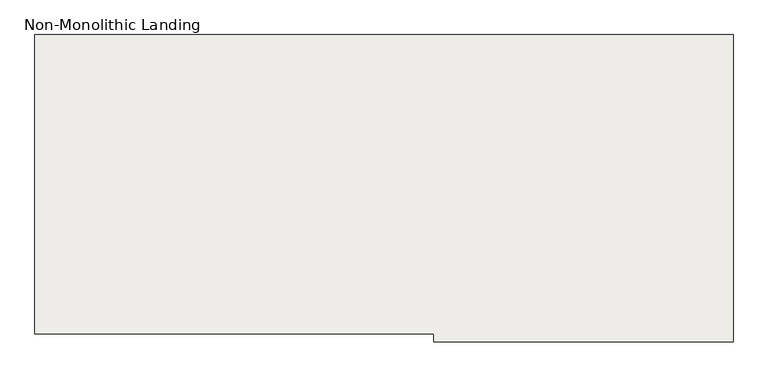
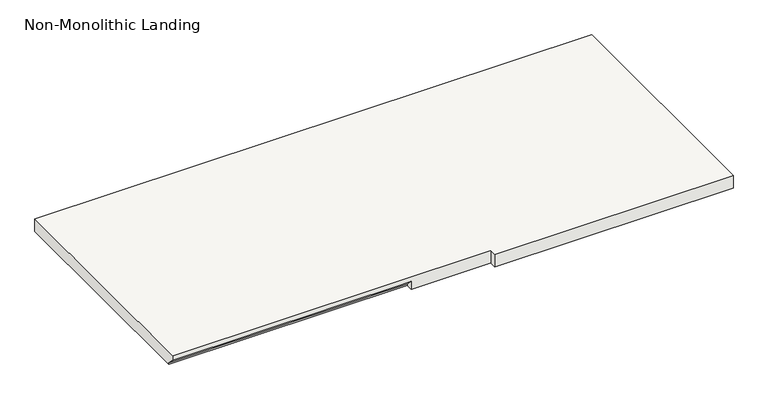
"""IFC4 building model written with IfcOpenShell, lengths in millimetres: slab geometry, Non-Monolithic Landing."""

from ifc_helpers import new_model, si_unit, origin, place, context, project, spatial, faceted_brep, source, transform, mapped, element, save


def non_monolithic_landing_55824b8c(model_context):
    return source(origin(), model_context, "Body", "Brep", [
        faceted_brep([(-3617.4415084, 23194.7216096, 45704.9005799), (-3617.4415084, 23220.1216096, 45679.5005799), (-2703.0415084, 23220.1216096, 45679.5005799), (-2703.0415084, 23194.7216096, 45704.9005799), (-2398.2415084, 23194.7216096, 45723.9505799), (-2398.2415084, 23169.3216096, 45723.9505799), (-1483.8415084, 23169.3216096, 45723.9505799), (-1483.8415084, 23194.7216096, 45723.9505799), (-1483.8415084, 24109.1216096, 45723.9505799), (-3617.4415084, 24109.1216096, 45723.9505799), (-3617.4415084, 23194.7216096, 45723.9505799), (-2703.0415084, 23220.1216096, 45673.1505799), (-3617.4415084, 23220.1216096, 45673.1505799), (-3617.4415084, 24109.1216096, 45673.1505799), (-1483.8415084, 24109.1216096, 45673.1505799), (-1483.8415084, 23194.7216096, 45673.1505799), (-1483.8415084, 23169.3216096, 45673.1505799), (-2398.2415084, 23169.3216096, 45673.1505799), (-2398.2415084, 23194.7216096, 45673.1505799), (-2703.0415084, 23194.7216096, 45673.1505799)], [[[0, 1, 2, 3]], [[4, 5, 6, 7, 8, 9, 10]], [[11, 12, 13, 14, 15, 16, 17, 18, 19]], [[12, 11, 2, 1]], [[11, 19, 3, 2]], [[4, 10, 0, 3, 19, 18]], [[5, 4, 18, 17]], [[6, 5, 17, 16]], [[7, 6, 16, 15]], [[8, 7, 15, 14]], [[9, 8, 14, 13]], [[10, 9, 13, 12, 1, 0]]]),
    ])


if __name__ == "__main__":
    model = new_model("IFC4")
    model_context = context("Model", 3, world=origin())
    ifc_project = project(units=[si_unit("LENGTHUNIT", "METRE", prefix="MILLI")], contexts=[model_context])
    site = spatial("IfcSite", under=ifc_project)
    building = spatial("IfcBuilding", under=site)
    placement = place(None, origin())
    non_monolithic_landing_shape = non_monolithic_landing_55824b8c(model_context)
    element("IfcSlab", 1, ObjectType="Non-Monolithic Landing", at=placement, inside=building, context=model_context, shape_type="MappedRepresentation", body=[
        mapped(non_monolithic_landing_shape, transform((0.0, 0.0, 0.0), x_axis=(1.0, 0.0, 0.0), y_axis=(0.0, 1.0, 0.0), z_axis=(0.0, 0.0, 1.0))),
    ])
    save(model, "model.ifc")
